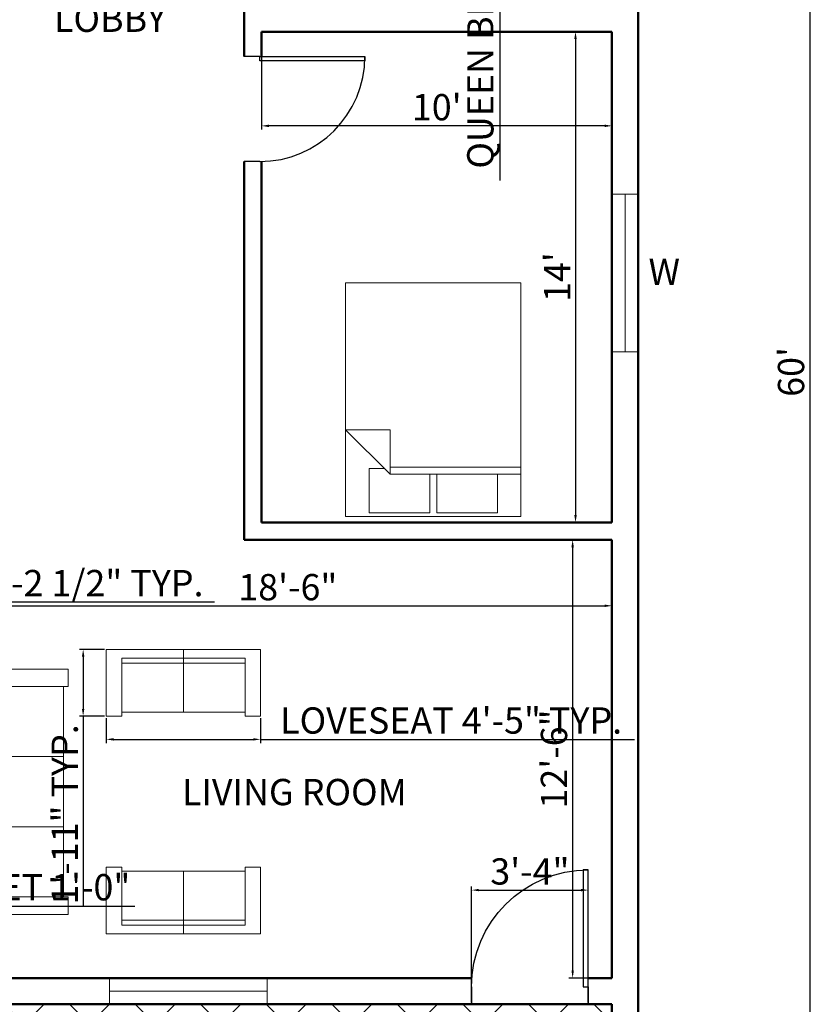
# Model space of a CAD drawing. Units: inches. Extents: x 3587 to 4539, y 1613 to 2440.
# Tile 5 of 8: x 3793 to 4067, y 1803 to 2140. Entities that reach past the tile are written whole.
import ezdxf

# ---------------------------------------------------------------- set-up
doc = ezdxf.new("R2010")
doc.units = ezdxf.units.IN
for name, color, linetype, lineweight in [('A-ANNO-DIMS', 2, 'Continuous', 18), ('A-ANNO-TEXT', 7, 'Continuous', 18), ('A-AREA-IDEN', 7, 'Continuous', 25), ('A-DOOR', 3, 'Continuous', 25), ('A-FLOR-PATT', 252, 'Continuous', 13), ('A-FURN', 8, 'Continuous', 18), ('A-GLAZ', 4, 'Continuous', 20), ('A-WALL', 7, 'Continuous', 50)]:
    doc.layers.add(name, color=color, linetype=linetype, lineweight=lineweight)
doc.styles.get("Standard").update_dxf_attribs({"font": 'arial.ttf'})
doc.dimstyles.new('ISO-25', dxfattribs={"dimtxt": 9, "dimasz": 2.5, "dimexe": 1.25, "dimexo": 0.625, "dimtad": 1, "dimlunit": 3, "dimtxsty": 'Standard', "dimcen": 2.5, "dimadec": 0, "dimazin": 0, "dimtfac": 1, "dimtmove": 0, "dimatfit": 3, "dimfxl": 1, "dimarcsym": 0})

# ---------------------------------------------------------------- blocks, each defined once
blk = doc.blocks.new('*U4')
for p, q in [((0, 0), (0, -6)), ((40, 0), (40, -6))]:
    blk.add_line(p, q)
blk.add_lwpolyline([(0, 0), (0, 40), (1.75, 40), (1.75, 0)], close=True)
blk.add_arc((0, 0), 40, 0, 90)
blk = doc.blocks.new('Bed - Queen')
for p, q in [((0, -80.00003), (0, 0)), ((0, 0), (59.99999, 0)), ((59.99999, 0), (59.99999, -80.00003)), ((7.99999, -1.2), (28.79998, -1.2)), ((7.99999, -14.4), (7.99999, -1.2)), ((28.79998, -1.2), (28.79998, -14.4)), ((31.19999, -1.2), (51.99999, -1.2)), ((31.19999, -14.4), (31.19999, -1.2)), ((51.99999, -1.2), (51.99999, -16.4)), ((0, -14.4), (44.8, -14.4)), ((44.8, -16.8), (0, -16.8)), ((59.99999, -29.6), (44.8, -14.4)), ((44.8, -14.4), (44.8, -29.6)), ((51.99999, -16.4), (46.79936, -16.4)), ((44.8, -29.6), (59.99999, -29.6)), ((59.99999, -80.00003), (0, -80.00003))]:
    blk.add_line(p, q)
blk = doc.blocks.new('*D23')
at = {"layer": 'A-ANNO-DIMS', "color": 0, "lineweight": -2, "transparency": 16777216}
for p, q in [((3875.52, 2135.31), (3875.52, 2102.45)), ((3995.52, 2135.31), (3995.52, 2102.45)), ((3993.02, 2103.7), (3878.02, 2103.7))]:
    blk.add_line(p, q, dxfattribs=at)
at = {"layer": 'A-ANNO-DIMS', "color": 0, "transparency": 16777216}
for points in [[(3878.02, 2104.12), (3878.02, 2103.28), (3875.52, 2103.7)], [(3993.02, 2104.12), (3993.02, 2103.28), (3995.52, 2103.7)]]:
    blk.add_solid(points, dxfattribs=at)
at = {"layer": 'Defpoints', "color": 0, "transparency": 16777216}
for p in [(3875.52, 2135.93), (3995.52, 2135.93), (3875.52, 2103.7)]:
    blk.add_point(p, dxfattribs=at)
at = {"layer": 'A-ANNO-DIMS', "color": 0, "transparency": 16777216, "insert": (3935.52, 2108.92), "char_height": 9, "attachment_point": 5}
blk.add_mtext("10'", dxfattribs=at)
blk = doc.blocks.new('*D24')
at = {"layer": 'A-ANNO-DIMS', "color": 0, "lineweight": -2, "transparency": 16777216}
for p, q in [((3994.9, 2135.93), (3981.79, 2135.93)), ((3983.04, 2133.43), (3983.04, 1970.43)), ((3994.9, 1967.93), (3981.79, 1967.93))]:
    blk.add_line(p, q, dxfattribs=at)
at = {"layer": 'A-ANNO-DIMS', "color": 0, "transparency": 16777216}
for points in [[(3982.62, 2133.43), (3983.46, 2133.43), (3983.04, 2135.93)], [(3982.62, 1970.43), (3983.46, 1970.43), (3983.04, 1967.93)]]:
    blk.add_solid(points, dxfattribs=at)
at = {"layer": 'Defpoints', "color": 0, "transparency": 16777216}
for p in [(3995.52, 2135.93), (3983.04, 1967.93), (3995.52, 1967.93)]:
    blk.add_point(p, dxfattribs=at)
at = {"layer": 'A-ANNO-DIMS', "color": 0, "transparency": 16777216, "insert": (3977.9, 2051.93), "char_height": 9, "attachment_point": 5, "rotation": 90}
blk.add_mtext("14'", dxfattribs=at)
blk = doc.blocks.new('*D26')
at = {"layer": 'A-ANNO-DIMS', "color": 0, "lineweight": -2, "transparency": 16777216}
for p, q in [((3994.9, 1961.93), (3980.8, 1961.93)), ((3982.05, 1959.43), (3982.05, 1814.43)), ((3994.9, 1811.93), (3980.8, 1811.93))]:
    blk.add_line(p, q, dxfattribs=at)
at = {"layer": 'A-ANNO-DIMS', "color": 0, "transparency": 16777216}
for points in [[(3981.64, 1959.43), (3982.47, 1959.43), (3982.05, 1961.93)], [(3981.64, 1814.43), (3982.47, 1814.43), (3982.05, 1811.93)]]:
    blk.add_solid(points, dxfattribs=at)
at = {"layer": 'Defpoints', "color": 0, "transparency": 16777216}
for p in [(3995.52, 1961.93), (3982.05, 1811.93), (3995.52, 1811.93)]:
    blk.add_point(p, dxfattribs=at)
at = {"layer": 'A-ANNO-DIMS', "color": 0, "transparency": 16777216, "insert": (3976.83, 1886.93), "char_height": 9, "attachment_point": 5, "rotation": 90}
blk.add_mtext('12\'-6"', dxfattribs=at)
blk = doc.blocks.new('*D27')
at = {"layer": 'A-ANNO-DIMS', "color": 0, "lineweight": -2, "transparency": 16777216}
for p, q in [((3773.52, 1812.56), (3773.52, 1940.63)), ((3776.02, 1939.38), (3993.02, 1939.38)), ((3995.52, 1812.56), (3995.52, 1940.63))]:
    blk.add_line(p, q, dxfattribs=at)
at = {"layer": 'A-ANNO-DIMS', "color": 0, "transparency": 16777216}
for points in [[(3776.02, 1939.8), (3776.02, 1938.96), (3773.52, 1939.38)], [(3993.02, 1939.8), (3993.02, 1938.96), (3995.52, 1939.38)]]:
    blk.add_solid(points, dxfattribs=at)
at = {"layer": 'Defpoints', "color": 0, "transparency": 16777216}
for p in [(3995.52, 1939.38), (3773.52, 1811.93), (3995.52, 1811.93)]:
    blk.add_point(p, dxfattribs=at)
at = {"layer": 'A-ANNO-DIMS', "color": 0, "transparency": 16777216, "insert": (3884.52, 1944.6), "char_height": 9, "attachment_point": 5}
blk.add_mtext('18\'-6"', dxfattribs=at)
blk = doc.blocks.new('*D28')
at = {"layer": 'A-ANNO-DIMS', "color": 0, "lineweight": -2, "transparency": 16777216}
for p, q in [((4087.49, 2372.93), (4061.98, 2372.93)), ((4063.23, 2370.43), (4063.23, 1655.43)), ((4087.49, 1652.93), (4061.98, 1652.93))]:
    blk.add_line(p, q, dxfattribs=at)
at = {"layer": 'A-ANNO-DIMS', "color": 0, "transparency": 16777216}
for points in [[(4062.81, 2370.43), (4063.65, 2370.43), (4063.23, 2372.93)], [(4062.81, 1655.43), (4063.65, 1655.43), (4063.23, 1652.93)]]:
    blk.add_solid(points, dxfattribs=at)
at = {"layer": 'Defpoints', "color": 0, "transparency": 16777216}
for p in [(4088.12, 2372.93), (4063.23, 1652.93), (4088.12, 1652.93)]:
    blk.add_point(p, dxfattribs=at)
at = {"layer": 'A-ANNO-DIMS', "color": 0, "transparency": 16777216, "insert": (4058.01, 2019.45), "char_height": 9, "attachment_point": 5, "rotation": 90}
blk.add_mtext("60'", dxfattribs=at)
blk = doc.blocks.new('SOFA-3-SEAT-84IN')
for p, q in [((0, 0), (0, 84)), ((26, 78), (3.47, 78)), ((3.47, 78), (3.47, 6)), ((5.38, 6), (5.38, 78)), ((24.44, 6), (24.44, 78)), ((24.44, 54), (0, 54)), ((24.44, 30), (0, 30)), ((26, 6), (3.47, 6))]:
    blk.add_line(p, q)
for points in [[(0, 84), (26, 84), (26, 78)], [(26, 6), (26, 0), (0, 0)]]:
    blk.add_lwpolyline(points)
blk = doc.blocks.new('LOVESEAT-2-SEAT')
for p, q in [((5.28, 22.88), (5.28, 3.05)), ((5.28, 21.51), (47.52, 21.51)), ((26.4, 21.51), (26.4, 0)), ((47.52, 22.88), (47.52, 3.05)), ((5.28, 4.74), (47.52, 4.74)), ((0, 0), (52.8, 0)), ((47.52, 3.05), (5.28, 3.05))]:
    blk.add_line(p, q)
for points in [[(5.28, 22.88), (0, 22.88), (0, 0)], [(52.8, 0), (52.8, 22.88), (47.52, 22.88)]]:
    blk.add_lwpolyline(points)
blk = doc.blocks.new('WINDOW-54IN')
for p, q in [((9, 54), (0, 54)), ((4.5, 54), (4.5, 0)), ((9, 0), (0, 0))]:
    blk.add_line(p, q)
blk = doc.blocks.new('*D60')
at = {"layer": 'A-ANNO-DIMS', "color": 0, "lineweight": -2, "transparency": 16777216}
for p, q in [((3945.78, 2301.11), (3958.4, 2301.11)), ((3957.15, 2298.61), (3957.15, 2223.61)), ((3945.78, 2221.11), (3958.4, 2221.11)), ((3957.15, 2221.11), (3957.15, 2084.97))]:
    blk.add_line(p, q, dxfattribs=at)
at = {"layer": 'A-ANNO-DIMS', "color": 0, "transparency": 16777216}
for points in [[(3956.74, 2298.61), (3957.57, 2298.61), (3957.15, 2301.11)], [(3956.74, 2223.61), (3957.57, 2223.61), (3957.15, 2221.11)]]:
    blk.add_solid(points, dxfattribs=at)
at = {"layer": 'Defpoints', "color": 0, "transparency": 16777216}
for p in [(3945.15, 2301.11), (3945.15, 2221.11), (3957.15, 2221.11)]:
    blk.add_point(p, dxfattribs=at)
at = {"layer": 'A-ANNO-DIMS', "color": 0, "transparency": 16777216, "insert": (3951.6, 2151.79), "char_height": 9, "attachment_point": 5, "rotation": 90}
blk.add_mtext('QUEEN BED 6\'-8" TYP.', dxfattribs=at)
blk = doc.blocks.new('*D62')
at = {"layer": 'A-ANNO-DIMS', "color": 0, "lineweight": -2, "transparency": 16777216}
for p, q in [((3822.34, 1900.94), (3822.34, 1892.39)), ((3875.15, 1900.94), (3875.15, 1892.39)), ((3824.84, 1893.64), (3872.65, 1893.64)), ((3875.15, 1893.64), (4003.23, 1893.64))]:
    blk.add_line(p, q, dxfattribs=at)
at = {"layer": 'A-ANNO-DIMS', "color": 0, "transparency": 16777216}
for points in [[(3824.84, 1894.06), (3824.84, 1893.23), (3822.34, 1893.64)], [(3872.65, 1894.06), (3872.65, 1893.23), (3875.15, 1893.64)]]:
    blk.add_solid(points, dxfattribs=at)
at = {"layer": 'Defpoints', "color": 0, "transparency": 16777216}
for p in [(3822.34, 1901.57), (3875.15, 1901.57), (3875.15, 1893.64)]:
    blk.add_point(p, dxfattribs=at)
at = {"layer": 'A-ANNO-DIMS', "color": 0, "transparency": 16777216, "insert": (3940.44, 1898.93), "char_height": 9, "attachment_point": 5}
blk.add_mtext('LOVESEAT 4\'-5" TYP.', dxfattribs=at)
blk = doc.blocks.new('*D63')
at = {"layer": 'A-ANNO-DIMS', "color": 0, "lineweight": -2, "transparency": 16777216}
for p, q in [((3821.72, 1924.45), (3813.17, 1924.45)), ((3814.42, 1921.95), (3814.42, 1904.07)), ((3821.72, 1901.57), (3813.17, 1901.57)), ((3814.42, 1901.57), (3814.42, 1836.81))]:
    blk.add_line(p, q, dxfattribs=at)
at = {"layer": 'A-ANNO-DIMS', "color": 0, "transparency": 16777216}
for points in [[(3814, 1921.95), (3814.84, 1921.95), (3814.42, 1924.45)], [(3814, 1904.07), (3814.84, 1904.07), (3814.42, 1901.57)]]:
    blk.add_solid(points, dxfattribs=at)
at = {"layer": 'Defpoints', "color": 0, "transparency": 16777216}
for p in [(3822.34, 1924.45), (3814.42, 1901.57), (3822.34, 1901.57)]:
    blk.add_point(p, dxfattribs=at)
at = {"layer": 'A-ANNO-DIMS', "color": 0, "transparency": 16777216, "insert": (3809.27, 1867.94), "char_height": 9, "attachment_point": 5, "rotation": 90}
blk.add_mtext('1\'-11" TYP.', dxfattribs=at)
blk = doc.blocks.new('*D72')
at = {"layer": 'A-ANNO-DIMS', "color": 0, "lineweight": -2, "transparency": 16777216}
for p, q in [((3739.17, 1837.74), (3739.17, 1835.32)), ((3751.17, 1837.74), (3751.17, 1835.32)), ((3741.67, 1836.57), (3748.67, 1836.57)), ((3751.17, 1836.57), (3832.12, 1836.57))]:
    blk.add_line(p, q, dxfattribs=at)
at = {"layer": 'A-ANNO-DIMS', "color": 0, "transparency": 16777216}
for points in [[(3741.67, 1836.98), (3741.67, 1836.15), (3739.17, 1836.57)], [(3748.67, 1836.98), (3748.67, 1836.15), (3751.17, 1836.57)]]:
    blk.add_solid(points, dxfattribs=at)
at = {"layer": 'Defpoints', "color": 0, "transparency": 16777216}
for p in [(3739.17, 1838.37), (3751.17, 1838.37), (3751.17, 1836.57)]:
    blk.add_point(p, dxfattribs=at)
at = {"layer": 'A-ANNO-DIMS', "color": 0, "transparency": 16777216, "insert": (3792.9, 1841.85), "char_height": 9, "attachment_point": 5}
blk.add_mtext('FAUCET 1\'-0"', dxfattribs=at)
blk = doc.blocks.new('*D78')
at = {"layer": 'A-ANNO-DIMS', "color": 0, "lineweight": -2, "transparency": 16777216}
for p, q in [((3693.28, 1942.22), (3693.28, 1939.45)), ((3707.6, 1942.22), (3707.6, 1939.45)), ((3695.78, 1940.7), (3705.1, 1940.7)), ((3707.6, 1940.7), (3859.36, 1940.7))]:
    blk.add_line(p, q, dxfattribs=at)
at = {"layer": 'A-ANNO-DIMS', "color": 0, "transparency": 16777216}
for points in [[(3695.78, 1941.11), (3695.78, 1940.28), (3693.28, 1940.7)], [(3705.1, 1941.11), (3705.1, 1940.28), (3707.6, 1940.7)]]:
    blk.add_solid(points, dxfattribs=at)
at = {"layer": 'Defpoints', "color": 0, "transparency": 16777216}
for p in [(3693.28, 1942.85), (3707.6, 1942.85), (3707.6, 1940.7)]:
    blk.add_point(p, dxfattribs=at)
at = {"layer": 'A-ANNO-DIMS', "color": 0, "transparency": 16777216, "insert": (3784.73, 1945.98), "char_height": 9, "attachment_point": 5}
blk.add_mtext('END CHAIR 1\'-2 1/2" TYP.', dxfattribs=at)
blk = doc.blocks.new('*D89')
at = {"layer": 'A-ANNO-DIMS', "color": 0, "lineweight": -2, "transparency": 16777216}
for p, q in [((3947.42, 1803.56), (3947.42, 1843.28)), ((3949.92, 1842.03), (3984.92, 1842.03)), ((3987.42, 1803.56), (3987.42, 1843.28))]:
    blk.add_line(p, q, dxfattribs=at)
at = {"layer": 'A-ANNO-DIMS', "color": 0, "transparency": 16777216}
for points in [[(3949.92, 1842.45), (3949.92, 1841.62), (3947.42, 1842.03)], [(3984.92, 1842.45), (3984.92, 1841.62), (3987.42, 1842.03)]]:
    blk.add_solid(points, dxfattribs=at)
at = {"layer": 'Defpoints', "color": 0, "transparency": 16777216}
for p in [(3987.42, 1842.03), (3947.42, 1802.93), (3987.42, 1802.93)]:
    blk.add_point(p, dxfattribs=at)
at = {"layer": 'A-ANNO-DIMS', "color": 0, "transparency": 16777216, "insert": (3967.42, 1847.26), "char_height": 9, "attachment_point": 5}
blk.add_mtext('3\'-4"', dxfattribs=at)

msp = doc.modelspace()

# ---------------------------------------------------------------- hatches: boundary and pattern name
at = {"layer": 'A-FLOR-PATT'}
h = msp.add_hatch(dxfattribs=at)
h.set_pattern_fill('ANSI37', color=256, scale=5)
h.paths.add_polyline_path([(3995.523, 1802.933), (3767.523, 1802.933), (3767.523, 1829.933), (3653.523, 1829.933), (3653.523, 1661.933), (3773.523, 1661.933), (3875.78, 1661.933), (3875.78, 1657.433), (3971.78, 1657.433), (3971.78, 1661.933), (3995.523, 1661.933)])
edge = h.paths.add_edge_path(flags=16)
edge.add_ellipse((-2931.215, 1767.797), major_axis=(-6663.992, 0), ratio=0.84230387, start_angle=179.6161332, end_angle=180.0902291, ccw=False)
edge.add_ellipse((3732.777, 1722.366), major_axis=(0.931, 0), ratio=0.8423039, start_angle=0, end_angle=90, ccw=False)
edge.add_line((3733.708, 1722.826), (3733.708, 1706.681))
edge.add_ellipse((3732.777, 1707.14), major_axis=(-0.931, 0), ratio=0.8423039, start_angle=90, end_angle=180, ccw=False)
edge.add_ellipse((-2931.215, 1767.797), major_axis=(-6663.992, 0), ratio=0.84230387, start_angle=179.3813568, end_angle=179.4717285, ccw=False)
edge.add_ellipse((3731.789, 1694.73), major_axis=(1.396, 0), ratio=0.8423039, start_angle=-0.62824, end_angle=68.46476, ccw=False)
edge.add_ellipse((-2931.681, 1767.797), major_axis=(-6665.43, 0), ratio=0.84230387, start_angle=179.3534459, end_angle=179.3717628, ccw=False)
edge.add_ellipse((3729.851, 1692.621), major_axis=(-3.3, 0), ratio=0.8423039, start_angle=90, end_angle=179.35345, ccw=False)
edge.add_line((3729.851, 1689.841), (3688.635, 1689.841))
edge.add_ellipse((3688.635, 1692.621), major_axis=(-3.3, 0), ratio=0.8423039, start_angle=0.64655, end_angle=90, ccw=False)
edge.add_ellipse((10350.167, 1767.797), major_axis=(-6665.43, 0), ratio=0.84230387, start_angle=0.6282372, end_angle=0.6465541, ccw=False)
edge.add_ellipse((3686.698, 1694.73), major_axis=(-1.396, 0), ratio=0.8423039, start_angle=-68.46476, end_angle=0.62824, ccw=False)
edge.add_ellipse((10349.701, 1767.797), major_axis=(-6663.992, 0), ratio=0.84230387, start_angle=0.5282715, end_angle=0.6465541, ccw=False)
edge.add_ellipse((3685.71, 1707.14), major_axis=(-0.931, 0), ratio=0.8423039, start_angle=0, end_angle=90, ccw=False)
edge.add_line((3684.779, 1706.681), (3684.779, 1722.826))
edge.add_ellipse((3685.71, 1722.366), major_axis=(-0.931, 0), ratio=0.8423039, start_angle=-90, end_angle=0, ccw=False)
edge.add_ellipse((10349.701, 1767.797), major_axis=(-6663.992, 0), ratio=0.84230387, start_angle=-0.0902291, end_angle=0.3838668, ccw=False)
edge.add_line((3685.721, 1778.291), (3685.164, 1778.291))
edge.add_ellipse((3685.71, 1779.075), major_axis=(0.931, 0), ratio=0.8423039, start_angle=180, end_angle=270, ccw=False)
edge.add_line((3684.779, 1779.075), (3684.779, 1794.761))
edge.add_ellipse((3685.71, 1794.301), major_axis=(-0.931, 0), ratio=0.8423039, start_angle=-90, end_angle=0, ccw=False)
edge.add_ellipse((4018.041, 1782.449), major_axis=(-332.308, 0), ratio=0.8423039, start_angle=-3.65043, end_angle=-2.17995, ccw=False)
edge.add_ellipse((3726.559, 1641.004), major_axis=(-197.1, 0), ratio=0.8423039, start_angle=-77.87403, end_angle=-76.21947, ccw=False)
edge.add_ellipse((3726.559, 1645.317), major_axis=(192.064, 0), ratio=0.8423039, start_angle=100.20954, end_angle=102.44463, ccw=False)
edge.add_ellipse((3676.281, 1937.008), major_axis=(-157.877, 0), ratio=0.8423039, start_angle=99.25657, end_angle=102.55493)
edge.add_line((3705.388, 1806.307), (3709.243, 1808.439))
edge.add_line((3709.243, 1808.439), (3713.098, 1806.307))
edge.add_ellipse((3742.206, 1937.008), major_axis=(157.877, 0), ratio=0.8423039, start_angle=257.44507, end_angle=260.74343)
edge.add_ellipse((3691.928, 1645.317), major_axis=(192.064, 0), ratio=0.8423039, start_angle=77.55537, end_angle=79.79046, ccw=False)
edge.add_ellipse((3691.928, 1641.004), major_axis=(197.1, 0), ratio=0.8423039, start_angle=76.21947, end_angle=77.87403, ccw=False)
edge.add_ellipse((3400.445, 1782.449), major_axis=(-332.308, 0), ratio=0.8423039, start_angle=182.17995, end_angle=183.65043, ccw=False)
edge.add_ellipse((3732.777, 1794.301), major_axis=(0.931, 0), ratio=0.8423039, start_angle=0, end_angle=90, ccw=False)
edge.add_line((3733.708, 1794.761), (3733.708, 1778.616))
edge.add_ellipse((3732.777, 1779.075), major_axis=(-0.931, 0), ratio=0.8423039, start_angle=90, end_angle=180, ccw=False)
edge = h.paths.add_edge_path(flags=0)
edge.add_ellipse((-2931.215, 1767.797), major_axis=(6663.061, 0), ratio=0.84230387, start_angle=-0.3777642, end_angle=-0.0555943, ccw=False)
edge.add_line((3731.642, 1723.866), (3729.234, 1733.318))
edge.add_ellipse((1402.768, 1748.102), major_axis=(2326.532, 0), ratio=0.84230387, start_angle=-0.364076, end_angle=0.120897)
edge.add_line((3729.293, 1753.011), (3731.841, 1761.332))
edge = h.paths.add_edge_path(flags=0)
edge.add_line((3729.082, 1764.306), (3727.708, 1754.004))
edge.add_ellipse((3711.004, 1714.253), major_axis=(-50.063, 0), ratio=0.8423039, start_angle=247.20809, end_angle=265.12993)
edge.add_line((3714.588, 1756.313), (3703.898, 1756.313))
edge.add_ellipse((3707.482, 1714.253), major_axis=(50.063, 0), ratio=0.8423039, start_angle=94.87007, end_angle=112.79191)
edge.add_line((3690.778, 1754.004), (3689.404, 1764.306))
edge.add_ellipse((3705.854, 1723.251), major_axis=(-51.443, 0), ratio=0.8423039, start_angle=-85.72258, end_angle=-68.16505, ccw=False)
edge.add_line((3702.619, 1766.496), (3715.867, 1766.496))
edge.add_ellipse((3712.632, 1723.251), major_axis=(-51.443, 0), ratio=0.8423039, start_angle=248.16505, end_angle=265.72258, ccw=False)
edge = h.paths.add_edge_path(flags=0)
edge.add_ellipse((3717.634, 1776.41), major_axis=(0.224, 3.988), ratio=0.6038336, start_angle=106.34259, end_angle=270.99799, ccw=False)
edge.add_line((3715.223, 1775.848), (3715.223, 1789.632))
edge.add_ellipse((3679.888, 1789.632), major_axis=(-35.335, 0), ratio=0.8423039, start_angle=180, end_angle=209.43857)
edge.add_ellipse((3738.598, 1789.632), major_axis=(35.335, 0), ratio=0.8423039, start_angle=150.56143, end_angle=180)
edge.add_line((3703.263, 1789.632), (3703.263, 1775.848))
edge.add_ellipse((3700.852, 1776.41), major_axis=(-0.224, 3.988), ratio=0.6038336, start_angle=89.00201, end_angle=253.65741, ccw=False)
edge.add_line((3698.442, 1776.317), (3698.442, 1785.634))
edge.add_line((3698.442, 1785.634), (3702.059, 1788.154))
edge.add_line((3702.059, 1788.154), (3703.263, 1788.154))
edge.add_line((3703.263, 1788.154), (3703.263, 1789.632))
edge.add_ellipse((3738.598, 1789.632), major_axis=(35.335, 0), ratio=0.8423039, start_angle=150.56143, end_angle=180, ccw=False)
edge.add_ellipse((3679.888, 1789.632), major_axis=(-35.335, 0), ratio=0.8423039, start_angle=180, end_angle=209.43857, ccw=False)
edge.add_line((3715.223, 1789.632), (3715.223, 1788.154))
edge.add_line((3715.223, 1788.154), (3716.427, 1788.154))
edge.add_line((3716.427, 1788.154), (3720.044, 1785.634))
edge.add_line((3720.044, 1785.634), (3720.044, 1776.317))
edge = h.paths.add_edge_path(flags=0)
edge.add_line((3727.708, 1721.281), (3727.708, 1709.439))
edge.add_ellipse((3709.243, 1785.774), major_axis=(92.488, 0), ratio=0.8423039, start_angle=256.40187, end_angle=283.59813, ccw=False)
edge.add_line((3690.778, 1709.439), (3690.778, 1721.281))
edge.add_ellipse((3709.243, 1797.616), major_axis=(92.488, 0), ratio=0.8423039, start_angle=256.40187, end_angle=283.59813)
edge = h.paths.add_edge_path(flags=0)
edge.add_line((3727.708, 1703.298), (3727.708, 1691.053))
edge.add_line((3727.708, 1691.053), (3690.778, 1691.053))
edge.add_line((3690.778, 1691.053), (3690.778, 1703.298))
edge.add_ellipse((3692.64, 1703.298), major_axis=(1.862, 0), ratio=0.8423039, start_angle=90, end_angle=180, ccw=False)
edge.add_line((3692.64, 1704.866), (3725.846, 1704.866))
edge.add_ellipse((3725.846, 1703.298), major_axis=(1.862, 0), ratio=0.8423039, start_angle=0, end_angle=90, ccw=False)
edge = h.paths.add_edge_path(flags=0)
edge.add_ellipse((6015.718, 1748.102), major_axis=(2326.532, 0), ratio=0.84230387, start_angle=179.879103, end_angle=180.364076)
edge.add_line((3689.252, 1733.318), (3686.845, 1723.866))
edge.add_ellipse((10349.701, 1767.797), major_axis=(6663.061, 0), ratio=0.84230387, start_angle=180.0555943, end_angle=180.3777642, ccw=False)
edge.add_line((3686.645, 1761.332), (3689.193, 1753.011))
h.paths.add_polyline_path([(3795.361, 1720.017), (3924.21, 1720.017), (3924.21, 1738.563), (3795.361, 1738.563)], flags=24)

# ---------------------------------------------------------------- linework, layer by layer
at = {"layer": 'A-WALL'}
for p, q in [((4004.523, 2372.933), (4004.523, 1652.933)), ((3869.523, 2213.933), (3869.523, 2135.933)), ((3869.523, 2135.933), (3869.523, 2127.481)), ((3995.523, 2135.933), (3875.523, 2135.933)), ((3875.523, 2135.933), (3875.523, 2127.481)), ((3995.523, 2135.933), (3995.523, 1967.933)), ((3869.523, 2091.481), (3869.523, 1961.933)), ((3875.523, 2091.486), (3875.523, 1967.933)), ((3995.523, 1967.933), (3875.523, 1967.933)), ((3995.523, 1961.933), (3869.523, 1961.933)), ((3995.523, 1961.933), (3995.523, 1811.933)), ((3947.532, 1811.933), (3773.523, 1811.933)), ((3995.523, 1811.933), (3987.42, 1811.933)), ((3995.523, 1802.933), (3767.523, 1802.933)), ((3995.523, 1802.933), (3995.523, 1661.933))]:
    msp.add_line(p, q, dxfattribs=at)

# ---------------------------------------------------------------- block references
at = {"layer": 'A-DOOR', "xscale": 0.9, "yscale": 0.9, "zscale": 0.9, "rotation": 270}
msp.add_blockref('*U4', (3874.923, 2127.481), dxfattribs=at)
at = {"layer": 'A-DOOR', "xscale": -1}
msp.add_blockref('*U4', (3987.42, 1808.933), dxfattribs=at)
at = {"layer": 'A-FURN', "rotation": 180}
msp.add_blockref('Bed - Queen', (3964.323, 1969.998), dxfattribs=at)
at = {"layer": 'A-FURN', "extrusion": (0, 0, -1), "zscale": -1, "rotation": 180}
msp.add_blockref('LOVESEAT-2-SEAT', (-3822.341, 1924.448), dxfattribs=at)
at = {"layer": 'A-FURN'}
for name, p in [('SOFA-3-SEAT-84IN', (3783.277, 1833.732)), ('LOVESEAT-2-SEAT', (3822.341, 1827.017))]:
    msp.add_blockref(name, p, dxfattribs=at)
at = {"layer": 'A-GLAZ'}
msp.add_blockref('WINDOW-54IN', (3995.523, 2026.316), dxfattribs=at)
at = {"layer": 'A-GLAZ', "rotation": 270}
msp.add_blockref('WINDOW-54IN', (3823.452, 1811.933), dxfattribs=at)

# ---------------------------------------------------------------- texts
at = {"layer": 'A-ANNO-TEXT', "insert": (4008.037, 2058.251), "char_height": 9, "attachment_point": 1}
msp.add_mtext_dynamic_manual_height_columns('W', width=47.85632, gutter_width=12.5, heights=[0], dxfattribs=at)
at = {"layer": 'A-AREA-IDEN', "char_height": 9, "attachment_point": 1}
for s, width, insert in [('LOBBY', 107.19817, (3804.425, 2144.864)), ('LIVING ROOM ', 173.2399, (3848.252, 1880.1))]:
    msp.add_mtext_dynamic_manual_height_columns(s, width=width, gutter_width=12.5, heights=[0], dxfattribs=dict(at, insert=insert))

# ---------------------------------------------------------------- dimensions: what is measured, and where the dimension line sits
at = {"layer": 'A-ANNO-DIMS'}
dim = msp.add_linear_dim(base=(4063.23, 1652.933), p1=(4088.116, 2372.933), p2=(4088.116, 1652.933), angle=90, dimstyle='ISO-25', override={"dimclrd": 0, "dimclre": 0, "dimclrt": 0}, dxfattribs=at)
dim.commit()
dim.dimension.update_dxf_attribs({"geometry": '*D28', "text_midpoint": (4063.23, 2019.453), "dimtype": 160})
for base, p1, p2, text, picture, middle in [((3957.153, 2221.11), (3945.153, 2301.11), (3945.153, 2221.11), 'QUEEN BED <> TYP.', '*D60', (3951.598, 2151.79)), ((3814.42, 1901.565), (3822.341, 1924.447), (3822.341, 1901.565), '<> TYP.', '*D63', (3809.273, 1867.938))]:
    dim = msp.add_linear_dim(base=base, p1=p1, p2=p2, angle=270, text=text, dimstyle='ISO-25', override={"dimdec": 1, "dimlfac": 1, "dimrnd": 0, "dimzin": 1, "dimdsep": 46, "dimlunit": 4, "dimfrac": 2}, dxfattribs=at)
    dim.commit()
    dim.dimension.update_dxf_attribs({"geometry": picture, "text_midpoint": middle})
for base, p1, p2, override, picture, middle in [((3875.523, 2103.698), (3995.523, 2135.933), (3875.523, 2135.933), {"dimclrd": 0, "dimclre": 0, "dimclrt": 0}, '*D23', (3935.523, 2108.919)), ((3995.523, 1939.381), (3773.523, 1811.933), (3995.523, 1811.933), {"dimclrd": 0, "dimclre": 0, "dimclrt": 0}, '*D27', (3884.523, 1944.601)), ((3987.42, 1842.033), (3947.42, 1802.933), (3987.42, 1802.933), {"dimdec": 1, "dimlfac": 1, "dimrnd": 0, "dimzin": 1, "dimdsep": 46, "dimlunit": 4, "dimfrac": 2}, '*D89', (3967.42, 1847.256))]:
    dim = msp.add_linear_dim(base=base, p1=p1, p2=p2, dimstyle='ISO-25', override=override, dxfattribs=at)
    dim.commit()
    dim.dimension.update_dxf_attribs({"geometry": picture, "text_midpoint": middle})
for base, p1, p2, picture, middle in [((3983.039, 1967.933), (3995.523, 2135.933), (3995.523, 1967.933), '*D24', (3977.895, 2051.933)), ((3982.055, 1811.933), (3995.523, 1961.933), (3995.523, 1811.933), '*D26', (3976.835, 1886.933))]:
    dim = msp.add_linear_dim(base=base, p1=p1, p2=p2, angle=90, dimstyle='ISO-25', override={"dimclrd": 0, "dimclre": 0, "dimclrt": 0}, dxfattribs=at)
    dim.commit()
    dim.dimension.update_dxf_attribs({"geometry": picture, "text_midpoint": middle})
for base, p1, p2, text, picture, middle in [((3707.598, 1940.698), (3693.278, 1942.846), (3707.598, 1942.846), 'END CHAIR <> TYP.', '*D78', (3784.728, 1945.976)), ((3875.146, 1893.644), (3822.341, 1901.565), (3875.146, 1901.565), 'LOVESEAT <> TYP.', '*D62', (3940.439, 1898.926)), ((3751.171, 1836.567), (3739.171, 1838.367), (3751.171, 1838.367), 'FAUCET <>', '*D72', (3792.896, 1841.846))]:
    dim = msp.add_linear_dim(base=base, p1=p1, p2=p2, text=text, dimstyle='ISO-25', override={"dimdec": 1, "dimlfac": 1, "dimrnd": 0, "dimzin": 1, "dimdsep": 46, "dimlunit": 4, "dimfrac": 2}, dxfattribs=at)
    dim.commit()
    dim.dimension.update_dxf_attribs({"geometry": picture, "text_midpoint": middle})

doc.saveas('drawing.dxf')
